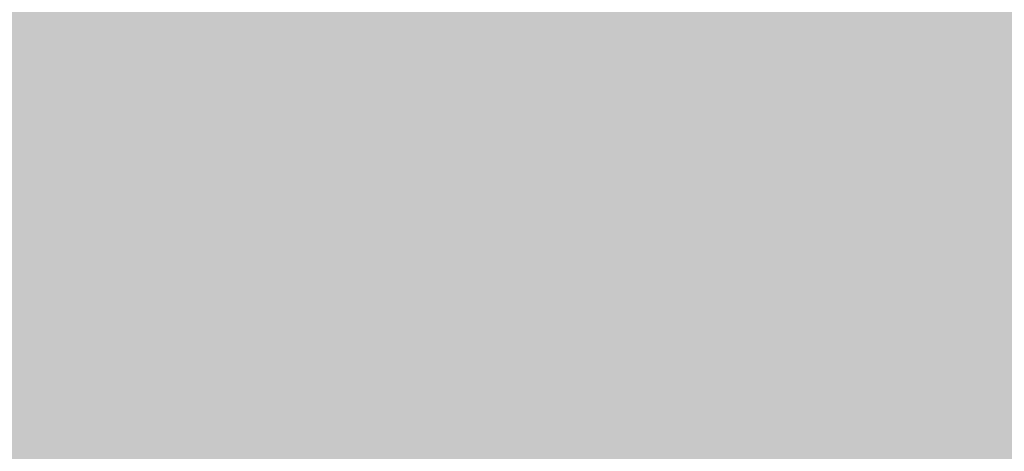
# Model space of a CAD drawing. Units: inches. Extents: x 2083 to 3317, y 1141 to 2115.
# Tile 148 of 256: x 3126.92826 to 3126.94671, y 1263.26594 to 1263.27402. Entities that reach past the tile are written whole.
import ezdxf

# ---------------------------------------------------------------- set-up
doc = ezdxf.new("R2010")
doc.units = ezdxf.units.IN
doc.layers.add('A-ANNO-DIMS', color=2, linetype='Continuous', lineweight=18)
doc.layers.add('A-WALL-PATT', color=251, linetype='Continuous', lineweight=13, true_color=0x636466)
doc.styles.get("Standard").update_dxf_attribs({"font": 'arial.ttf'})
doc.dimstyles.new('ISO-25', dxfattribs={"dimtxt": 12, "dimasz": 12, "dimexe": 1.25, "dimexo": 0.625, "dimtad": 1, "dimlunit": 3, "dimtxsty": 'Standard', "dimcen": 2.5, "dimadec": 0, "dimazin": 0, "dimtfac": 1, "dimtmove": 0, "dimatfit": 3, "dimfxl": 1, "dimarcsym": 0})

# ---------------------------------------------------------------- blocks, each defined once
blk = doc.blocks.new('*D26')
at = {"layer": 'A-ANNO-DIMS', "color": 0, "lineweight": -2, "transparency": 16777216}
for p, q in [((3088.985844, 1274.915092), (3088.985844, 1270.951963)), ((3111.240037, 1274.915092), (3111.240037, 1270.951963)), ((3076.985844, 1272.201963), (2840.262447, 1272.201963)), ((3111.240037, 1272.201963), (3088.985844, 1272.201963)), ((3123.240037, 1272.201963), (3135.240037, 1272.201963))]:
    blk.add_line(p, q, dxfattribs=at)
at = {"layer": 'A-ANNO-DIMS', "color": 0, "transparency": 16777216}
for points in [[(3076.985844, 1274.201963), (3076.985844, 1270.201963), (3088.985844, 1272.201963)], [(3123.240037, 1274.201963), (3123.240037, 1270.201963), (3111.240037, 1272.201963)]]:
    blk.add_solid(points, dxfattribs=at)
at = {"layer": 'Defpoints', "color": 0, "transparency": 16777216}
for p in [(3088.985844, 1275.540092), (3111.240037, 1275.540092), (3088.985844, 1272.201963)]:
    blk.add_point(p, dxfattribs=at)
at = {"layer": 'A-ANNO-DIMS', "color": 0, "transparency": 16777216, "insert": (2952.624146, 1279.031602), "char_height": 12, "attachment_point": 5}
blk.add_mtext('NIGHTSTAND 1\'-10 1/2" TYP.', dxfattribs=at)
blk = doc.blocks.new('*D27')
at = {"layer": 'A-ANNO-DIMS', "color": 0, "lineweight": -2, "transparency": 16777216}
for p, q in [((3114.578165, 1309.794285), (3114.578165, 1321.794285)), ((3111.865037, 1297.794285), (3115.828165, 1297.794285)), ((3114.578165, 1297.794285), (3114.578165, 1275.540092)), ((3111.865037, 1275.540092), (3115.828165, 1275.540092)), ((3114.578165, 1263.540092), (3114.578165, 1140.988591))]:
    blk.add_line(p, q, dxfattribs=at)
at = {"layer": 'A-ANNO-DIMS', "color": 0, "transparency": 16777216}
for points in [[(3112.578165, 1309.794285), (3116.578165, 1309.794285), (3114.578165, 1297.794285)], [(3112.578165, 1263.540092), (3116.578165, 1263.540092), (3114.578165, 1275.540092)]]:
    blk.add_solid(points, dxfattribs=at)
at = {"layer": 'Defpoints', "color": 0, "transparency": 16777216}
for p in [(3111.240037, 1297.794285), (3111.240037, 1275.540092), (3114.578165, 1275.540092)]:
    blk.add_point(p, dxfattribs=at)
at = {"layer": 'A-ANNO-DIMS', "color": 0, "transparency": 16777216, "insert": (3107.748527, 1196.264342), "char_height": 12, "attachment_point": 5, "rotation": 90}
blk.add_mtext('1\'-10 1/2" TYP.', dxfattribs=at)

msp = doc.modelspace()

# ---------------------------------------------------------------- hatches: boundary and pattern name
at = {"layer": 'A-WALL-PATT'}
h = msp.add_hatch(color=256, dxfattribs=at)
h.dxf.hatch_style = 1
h.paths.add_polyline_path([(3126.959783, 2020.76136), (2748.959783, 2020.76136), (2604.959783, 2020.76136), (2226.959783, 2020.76136), (2226.959783, 1702.76136), (2466.959783, 1702.76136), (2466.959783, 1582.76136), (2418.959783, 1582.76136), (2418.959783, 1477.76136), (2226.959783, 1477.76136), (2226.959783, 1263.26136), (2544.959783, 1263.26136), (2544.959783, 1411.76136), (2604.959783, 1411.76136), (2685.959783, 1411.76136), (2685.959783, 1420.76136), (2604.959783, 1420.76136), (2604.959783, 1573.76136), (2604.959783, 1702.76136), (2604.959783, 2011.76136), (2748.959783, 2011.76136), (2748.959783, 1702.76136), (2862.959783, 1702.76136), (2862.959783, 1621.76136), (2871.959783, 1621.76136), (2871.959783, 1702.76136), (2883.959783, 1702.76136), (2883.959783, 1706.939459, -0.026459), (2883.959783, 1711.76136), (2757.959783, 1711.76136), (2757.959783, 1807.76136), (2787.959783, 1807.76136), (2787.959783, 1812.26136), (2757.959783, 1812.26136), (2757.959783, 2011.76136), (2877.959783, 2011.76136), (2877.959783, 1812.26136), (2847.959783, 1812.26136), (2847.959783, 1807.76136), (2889.835742, 1807.76136), (2889.835742, 1812.26136), (2882.459783, 1812.26136), (2882.459783, 2011.76136), (3117.959783, 2011.76136), (3117.959783, 1812.26136), (2937.835742, 1812.26136), (2937.835742, 1807.76136), (2995.709783, 1807.76136), (2995.709783, 1796.117666), (3000.209783, 1796.117666), (3000.209783, 1807.76136), (3117.959783, 1807.76136), (3117.959783, 1711.76136), (3000.209783, 1711.76136), (3000.209783, 1760.117666), (2998.572705, 1760.117666, -0.020711), (2995.709783, 1760.117666), (2995.709783, 1711.76136), (2931.959783, 1711.76136), (2931.959783, 1702.76136), (3126.959783, 1702.76136)])
h.paths.add_polyline_path([(2471.459783, 2011.76136), (2471.459783, 1810.01136), (2462.716936, 1810.01136), (2462.716936, 1805.51136), (2505.959783, 1805.51136), (2505.959783, 1810.01136), (2475.959783, 1810.01136), (2475.959783, 2011.76136), (2595.959783, 2011.76136), (2595.959783, 1810.01136), (2565.959783, 1810.01136), (2565.959783, 1805.51136), (2595.959783, 1805.51136), (2595.959783, 1711.76136), (2235.959783, 1711.76136), (2235.959783, 1805.51136), (2353.709783, 1805.51136), (2353.709783, 1796.054162), (2358.209783, 1796.054162), (2358.209783, 1805.51136), (2414.716936, 1805.51136), (2414.716936, 1810.01136), (2235.959783, 1810.01136), (2235.959783, 2011.76136)], flags=16)
h.paths.add_polyline_path([(2270.204734, 1994.610008), (2270.204734, 1970.610008), (2246.204734, 1970.610008), (2246.204734, 1994.610008)], flags=0)
edge = h.paths.add_edge_path(flags=0)
edge.add_ellipse((2332.027391, 1899.798176), major_axis=(-3.042994, 3.042994), ratio=0.16825245, start_angle=-161.332166, end_angle=-156.307114, ccw=False)
edge.add_ellipse((2333.082037, 1898.74353), major_axis=(-1.054646, 1.054646), ratio=0.4535321, start_angle=-123.371019, end_angle=-94.159107)
edge = h.paths.add_edge_path(flags=0)
edge.add_ellipse((2332.027391, 1968.87629), major_axis=(3.042994, 3.042994), ratio=0.16825245, start_angle=18.667834, end_angle=23.692886)
edge.add_spline(control_points=[(2332.925596, 1970.691105), (2332.226768, 1970.3361), (2330.893709, 1969.658905), (2328.41308, 1970.932138), (2327.203934, 1967.748712), (2324.709596, 1969.955589), (2322.532822, 1967.012354), (2320.012846, 1971.295812), (2317.680308, 1968.157845), (2316.040526, 1967.102047), (2315.426904, 1966.809602)], knot_values=[0, 0, 0, 0, 2.267059, 4.324559, 6.685584, 8.878641, 11.121502, 14.300359, 17.755284, 19.732645, 19.732645, 19.732645, 19.732645], degree=3, periodic=0)
edge.add_ellipse((2332.027391, 1968.87629), major_axis=(3.042994, 3.042994), ratio=0.16825245, start_angle=18.667834, end_angle=23.692886, ccw=False)
edge.add_ellipse((2333.082037, 1969.930936), major_axis=(1.054646, 1.054646), ratio=0.4535321, start_angle=56.628981, end_angle=85.840893, ccw=False)
edge = h.paths.add_edge_path(flags=0)
edge.add_spline(control_points=[(2296.428287, 1967.987908), (2293.627804, 1965.336314), (2287.703624, 1959.727094), (2299.74386, 1949.995699), (2294.532591, 1935.668528), (2290.573228, 1920.603512), (2293.394124, 1909.973691), (2296.185407, 1904.966543)], knot_values=[0.099185, 0.099185, 0.099185, 0.099185, 0.345301, 0.619822, 0.982653, 1.386093, 1.810555, 1.810555, 1.810555, 1.810555], degree=3, periodic=0)
edge.add_spline(control_points=[(2296.185407, 1904.966543), (2297.383582, 1902.6193), (2298.000969, 1901.949312), (2298.55297, 1901.468155)], knot_values=[0.006246, 0.006246, 0.006246, 0.006246, 0.055476, 0.055476, 0.055476, 0.055476], degree=3, periodic=0)
edge.add_spline(control_points=[(2298.55297, 1901.468155), (2297.258612, 1900.923224), (2295.225294, 1900.232126), (2293.060229, 1900.614205), (2292.101423, 1900.788415), (2292.089578, 1900.790568)], knot_values=[0.312835, 0.312835, 0.312835, 0.312835, 0.40178, 0.474987, 0.475903, 0.475903, 0.475903, 0.475903], degree=3, periodic=0)
edge.add_arc((2292.793646, 1904.664109), 3.937008, 215.420897, 259.698179, ccw=False)
edge.add_spline(control_points=[(2289.585314, 1902.382304), (2289.476652, 1902.535087), (2289.36848, 1902.688035), (2289.260865, 1902.84117)], knot_values=[0.102872, 0.102872, 0.102872, 0.102872, 0.116896, 0.116896, 0.116896, 0.116896], degree=3, periodic=0)
edge.add_spline(control_points=[(2289.260865, 1902.84117), (2288.686604, 1902.550192), (2287.640048, 1902.019902), (2285.881337, 1901.873954), (2283.852972, 1901.504352), (2281.719987, 1899.710538), (2278.466991, 1899.492942), (2276.157136, 1901.883202), (2272.258953, 1899.804071), (2267.777605, 1901.843183), (2262.243882, 1900.184033), (2257.414927, 1901.782061), (2254.318374, 1900.72612), (2253.178285, 1900.337343)], knot_values=[0, 0, 0, 0, 1.907977, 3.477176, 5.261074, 7.972851, 11.680248, 13.717921, 16.939592, 22.789562, 27.502503, 33.595215, 37.145618, 37.145618, 37.145618, 37.145618], degree=3, periodic=0)
edge.add_line((2253.178285, 1900.337343), (2250.24424, 1902.84117))
edge.add_line((2250.24424, 1902.84117), (2250.24424, 1965.833296))
edge.add_line((2250.24424, 1965.833296), (2253.178285, 1968.337123))
edge.add_spline(control_points=[(2253.178285, 1968.337123), (2254.318374, 1967.948346), (2257.414927, 1966.892405), (2262.243882, 1968.490433), (2267.777605, 1966.831283), (2271.52673, 1968.537217), (2273.875914, 1967.828289), (2274.206701, 1967.727642)], knot_values=[0, 0, 0, 0, 0.09018, 0.244935, 0.364644, 0.513233, 0.537855, 0.537855, 0.537855, 0.537855], degree=3, periodic=0)
edge.add_arc((2274.352887, 1963.793349), 3.937008, 72.051134, 92.127949, ccw=False)
edge.add_arc((2281.296933, 1985.230003), 18.596298, 252.0511336, 288.5657217)
edge.add_arc((2292.316717, 1956.02888), 12.646081, 71.0267879, 113.7782184, ccw=False)
edge = h.paths.add_edge_path(flags=0)
edge.add_spline(control_points=[(2274.899415, 1951.856195), (2275.066156, 1951.616592), (2275.232687, 1951.376588), (2275.397987, 1951.135855)], knot_values=[1.409916, 1.409916, 1.409916, 1.409916, 1.43159, 1.43159, 1.43159, 1.43159], degree=3, periodic=0)
edge.add_spline(control_points=[(2275.397987, 1951.135855), (2275.792106, 1950.561885), (2276.179231, 1949.983774), (2276.545546, 1949.397103)], knot_values=[1.358238, 1.358238, 1.358238, 1.358238, 1.409916, 1.409916, 1.409916, 1.409916], degree=3, periodic=0)
edge.add_line((2276.545546, 1949.397103), (2277.437289, 1947.862185))
edge.add_spline(control_points=[(2277.437289, 1947.862185), (2276.303834, 1945.673115), (2274.639698, 1942.426882), (2274.631615, 1938.0939), (2272.799124, 1930.85155), (2274.356426, 1943.897046), (2275.947681, 1947.923356), (2276.545546, 1949.397103)], knot_values=[0.005632, 0.005632, 0.005632, 0.005632, 0.186014, 0.266002, 0.357087, 0.59639, 0.739732, 0.739732, 0.739732, 0.739732], degree=3, periodic=0)
edge.add_spline(control_points=[(2276.545546, 1949.397103), (2276.179231, 1949.983774), (2275.792106, 1950.561885), (2275.397987, 1951.135855)], knot_values=[1.358238, 1.358238, 1.358238, 1.358238, 1.409916, 1.409916, 1.409916, 1.409916], degree=3, periodic=0)
edge.add_spline(control_points=[(2275.397987, 1951.135855), (2274.9425, 1950.080452), (2274.20776, 1948.025272), (2273.934602, 1944.851477), (2272.468534, 1937.627489), (2273.466216, 1945.696466), (2274.700615, 1951.059472), (2274.899415, 1951.856195)], knot_values=[0.104364, 0.104364, 0.104364, 0.104364, 0.189636, 0.269624, 0.36071, 0.600013, 0.644622, 0.644622, 0.644622, 0.644622], degree=3, periodic=0)
h.paths.add_polyline_path([(2269.167514, 1963.127573, -0.357527), (2268.170633, 1960.97637, -0.092561), (2268.170633, 1939.436325, -0.357527), (2269.167514, 1937.285122, -0.357527), (2267.01631, 1938.282002, -0.164785), (2254.685581, 1938.282002, -0.357527), (2252.534378, 1937.285122, -0.357527), (2253.531259, 1939.436325, -0.092561), (2253.531259, 1960.97637, -0.357527), (2252.534378, 1963.127573, -0.357527), (2254.685581, 1962.130692, -0.164785), (2267.01631, 1962.130692, -0.357527)], flags=0)
h.paths.add_polyline_path([(2248.874068, 1967.8018), (2248.874068, 1957.02771), (2249.457783, 1957.02771), (2249.457783, 1911.646756), (2248.874068, 1911.646756), (2248.874068, 1900.872666), (2246.511863, 1900.872666, 0.197327), (2244.149658, 1902.456873), (2244.149658, 1966.217592, 0.197327), (2246.511863, 1967.8018)], flags=0)
h.paths.add_polyline_path([(2269.167514, 1931.389344, -0.357527), (2268.170633, 1929.238141, -0.092561), (2268.170633, 1907.698096, -0.357527), (2269.167514, 1905.546893, -0.357527), (2267.01631, 1906.543774, -0.164785), (2254.685581, 1906.543774, -0.357527), (2252.534378, 1905.546893, -0.357527), (2253.531259, 1907.698096, -0.092561), (2253.531259, 1929.238141, -0.357527), (2252.534378, 1931.389344, -0.357527), (2254.685581, 1930.392463, -0.164785), (2267.01631, 1930.392463, -0.357527)], flags=0)
edge = h.paths.add_edge_path(flags=0)
edge.add_spline(control_points=[(2276.196858, 1906.723702), (2276.168144, 1909.028928), (2276.114049, 1913.371852), (2270.598417, 1924.924978), (2273.905175, 1919.012779), (2275.921711, 1916.262063), (2275.47457, 1912.402149), (2277.257874, 1910.380621), (2276.696044, 1908.225036), (2276.646218, 1906.813023), (2276.617825, 1906.008407)], knot_values=[0, 0, 0, 0, 8.61026, 16.221274, 18.843057, 23.804898, 27.440828, 29.356102, 31.203478, 33.650687, 33.650687, 33.650687, 33.650687], degree=3, periodic=0)
edge.add_spline(control_points=[(2276.617825, 1906.008407), (2276.623313, 1905.624144), (2276.497738, 1904.628661), (2275.441779, 1903.854725), (2274.937314, 1903.08045), (2274.85908, 1902.84117)], knot_values=[0.156488, 0.156488, 0.156488, 0.156488, 0.184398, 0.231376, 0.250598, 0.250598, 0.250598, 0.250598], degree=3, periodic=0)
edge.add_line((2274.85908, 1902.84117), (2276.50598, 1902.84117))
edge.add_spline(control_points=[(2276.50598, 1902.84117), (2276.788308, 1903.08494), (2277.665071, 1904.125196), (2278.249538, 1904.340738), (2277.653872, 1908.527387), (2278.15567, 1906.227808), (2278.100464, 1905.285948), (2278.846675, 1904.069005), (2277.856785, 1903.414948), (2277.874191, 1902.99105), (2277.903562, 1902.84117)], knot_values=[0.059574, 0.059574, 0.059574, 0.059574, 0.080753, 0.103741, 0.16972, 0.176036, 0.207137, 0.240474, 0.262341, 0.27366, 0.27366, 0.27366, 0.27366], degree=3, periodic=0)
edge.add_line((2277.903562, 1902.84117), (2280.029825, 1902.84117))
edge.add_spline(control_points=[(2280.029825, 1902.84117), (2279.888221, 1903.088398), (2279.499257, 1903.981551), (2280.152284, 1905.939349), (2278.103615, 1909.657757), (2279.762395, 1907.185285), (2280.3279, 1904.874861), (2280.485109, 1903.48959), (2281.463269, 1903.249432), (2281.758343, 1902.936497), (2281.834036, 1902.84117)], knot_values=[0.013856, 0.013856, 0.013856, 0.013856, 0.034874, 0.088867, 0.107879, 0.126738, 0.158714, 0.193757, 0.217487, 0.226722, 0.226722, 0.226722, 0.226722], degree=3, periodic=0)
edge.add_spline(control_points=[(2281.834036, 1902.84117), (2281.787535, 1902.826703), (2281.647022, 1902.782988), (2281.395527, 1902.85949), (2281.088077, 1902.985242), (2280.720683, 1903.060902), (2280.333451, 1903.025726), (2280.124767, 1902.898879), (2280.029825, 1902.84117)], knot_values=[0, 0, 0, 0, 0.14413, 0.435517, 0.749276, 1.153046, 1.548371, 1.878348, 1.878348, 1.878348, 1.878348], degree=3, periodic=0)
edge.add_line((2280.029825, 1902.84117), (2277.903562, 1902.84117))
edge.add_spline(control_points=[(2277.903562, 1902.84117), (2277.892855, 1902.795855), (2277.865396, 1902.679637), (2277.607479, 1902.687483), (2277.27405, 1902.8007), (2276.837921, 1902.619775), (2276.583807, 1902.789261), (2276.50598, 1902.84117)], knot_values=[0, 0, 0, 0, 0.127189, 0.326199, 0.628009, 1.24357, 1.515331, 1.515331, 1.515331, 1.515331], degree=3, periodic=0)
edge.add_line((2276.50598, 1902.84117), (2274.85908, 1902.84117))
edge.add_spline(control_points=[(2274.85908, 1902.84117), (2274.814437, 1902.898587), (2274.72513, 1903.013446), (2274.493477, 1903.118968), (2274.244285, 1902.960539), (2273.937121, 1903.184942), (2273.614039, 1902.983143), (2273.408316, 1902.883045), (2273.322254, 1902.84117)], knot_values=[0, 0, 0, 0, 0.21843, 0.436957, 0.687977, 0.990379, 1.398396, 1.69185, 1.69185, 1.69185, 1.69185], degree=3, periodic=0)
edge.add_spline(control_points=[(2273.322254, 1902.84117), (2273.61674, 1903.445692), (2274.273998, 1904.538253), (2276.027239, 1904.573702), (2276.206963, 1906.583637), (2276.196858, 1906.723702)], knot_values=[0.012227, 0.012227, 0.012227, 0.012227, 0.059472, 0.106218, 0.134458, 0.134458, 0.134458, 0.134458], degree=3, periodic=0)
h.paths.add_polyline_path([(2270.776054, 1897.789828), (2270.776054, 1873.789828), (2246.776054, 1873.789828), (2246.776054, 1897.789828)], flags=0)
h.paths.add_polyline_path([(2353.709783, 1760.005059), (2353.709783, 1760.054162), (2358.209783, 1760.054162, -0.033729)], flags=0)
h.paths.add_polyline_path([(2321.819119, 1737.529186), (2341.995327, 1737.529186, -0.414214), (2343.203273, 1736.321241), (2343.203273, 1721.020596, -0.414214), (2341.995327, 1719.812651), (2321.819119, 1719.812651, -0.414214), (2320.611173, 1721.020596), (2320.611173, 1736.321241, -0.414214)], flags=0)
h.paths.add_polyline_path([(2324.23501, 1736.321241), (2339.579436, 1736.321241, -0.414214), (2341.995327, 1733.905349), (2341.995327, 1725.44973, -0.414214), (2339.579436, 1723.033839), (2333.680588, 1723.033839), (2333.845317, 1722.045467, -0.870646), (2335.425399, 1721.825893, -0.767327), (2333.922694, 1721.423245), (2331.291024, 1721.423245, -0.767327), (2329.788319, 1721.825893, -0.870646), (2331.368401, 1722.045467), (2331.53313, 1723.033839), (2324.23501, 1723.033839, -0.414214), (2321.819119, 1725.44973), (2321.819119, 1733.905349, -0.414214)], flags=0)
h.paths.add_polyline_path([(2570.483789, 1928.615444), (2589.683789, 1928.615444), (2590.168829, 1928.615444), (2590.168829, 1904.993397), (2570.483789, 1904.993397)], flags=0)
h.paths.add_polyline_path([(2574.447324, 1927.263822, -1), (2572.828836, 1927.263822, -1)], flags=0)
h.paths.add_polyline_path([(2573.089867, 1926.940877), (2573.925032, 1927.776042), (2574.147743, 1927.553332), (2573.312577, 1926.718166)], flags=0)
h.paths.add_polyline_path([(2578.779065, 1919.729618, -1), (2571.591663, 1919.729618, -1)], flags=0)
h.paths.add_polyline_path([(2578.385364, 1919.729618, -1), (2571.985364, 1919.729618, -1)], flags=0)
h.paths.add_polyline_path([(2331.595764, 1729.476216, -1), (2333.617954, 1729.476216, -1)], flags=0)
h.paths.add_polyline_path([(2578.034228, 1927.263822, -1), (2576.41574, 1927.263822, -1)], flags=0)
h.paths.add_polyline_path([(2576.688851, 1927.531089), (2576.911562, 1927.753799), (2577.746728, 1926.918634), (2577.524017, 1926.695923)], flags=0)
h.paths.add_polyline_path([(2578.139065, 1909.859539, -1), (2572.231663, 1909.859539, -1)], flags=0)
h.paths.add_polyline_path([(2577.745364, 1909.859539, -1), (2572.625364, 1909.859539, -1)], flags=0)
h.paths.add_polyline_path([(2583.797718, 1927.263822, -1), (2582.179229, 1927.263822, -1)], flags=0)
h.paths.add_polyline_path([(2582.718649, 1927.753799), (2583.553814, 1926.918634), (2583.331103, 1926.695923), (2582.495938, 1927.531089)], flags=0)
h.paths.add_polyline_path([(2582.495938, 1927.531089), (2582.718649, 1927.753799), (2583.553814, 1926.918634), (2583.331103, 1926.695923)], flags=0)
h.paths.add_polyline_path([(2587.739065, 1920.529618, -1), (2581.831663, 1920.529618, -1)], flags=0)
h.paths.add_polyline_path([(2587.345364, 1920.529618, -1), (2582.225364, 1920.529618, -1)], flags=0)
h.paths.add_polyline_path([(2587.384622, 1927.263822, -1), (2585.766133, 1927.263822, -1)], flags=0)
h.paths.add_polyline_path([(2586.081993, 1926.980247), (2586.917158, 1927.815412), (2587.139869, 1927.592702), (2586.304703, 1926.757536)], flags=0)
h.paths.add_polyline_path([(2588.379065, 1910.659539, -1), (2581.191663, 1910.659539, -1)], flags=0)
h.paths.add_polyline_path([(2587.985364, 1910.659539, -1), (2581.585364, 1910.659539, -1)], flags=0)
h.paths.add_polyline_path([(2417.167729, 1729.477895), (2437.343937, 1729.477895, -0.414214), (2438.551883, 1728.26995), (2438.551883, 1712.969306, -0.414214), (2437.343937, 1711.76136), (2417.167729, 1711.76136, -0.414214), (2415.959783, 1712.969306), (2415.959783, 1728.26995, -0.414214)], flags=0)
h.paths.add_polyline_path([(2419.58362, 1728.26995), (2434.928046, 1728.26995, -0.414214), (2437.343937, 1725.854059), (2437.343937, 1717.39844, -0.414214), (2434.928046, 1714.982548), (2429.029199, 1714.982548), (2429.193927, 1713.994176, -0.870646), (2430.774009, 1713.774603, -0.767327), (2429.271304, 1713.371954), (2426.639634, 1713.371954, -0.767327), (2425.136929, 1713.774603, -0.870646), (2426.717011, 1713.994176), (2426.88174, 1714.982548), (2419.58362, 1714.982548, -0.414214), (2417.167729, 1717.39844), (2417.167729, 1725.854059, -0.414214)], flags=0)
h.paths.add_polyline_path([(2419.58362, 1728.26995), (2434.928046, 1728.26995, -0.414214), (2437.343937, 1725.854059), (2437.343937, 1717.39844, -0.414214), (2434.928046, 1714.982548), (2429.029199, 1714.982548), (2428.358118, 1719.009034), (2427.552821, 1719.009034), (2426.88174, 1714.982548), (2419.58362, 1714.982548, -0.414214), (2417.167729, 1717.39844), (2417.167729, 1725.854059, -0.414214)], flags=0)
h.paths.add_polyline_path([(2426.944374, 1721.424925, -1), (2428.966564, 1721.424925, -1)], flags=0)
h.paths.add_polyline_path([(2475.959783, 1702.76136), (2595.959783, 1702.76136), (2595.959783, 1582.76136), (2475.959783, 1582.76136)], flags=16)
h.paths.add_polyline_path([(2427.959783, 1573.76136), (2595.959783, 1573.76136), (2595.959783, 1468.76136), (2595.959783, 1420.76136), (2384.459783, 1420.76136), (2384.459783, 1468.76136), (2427.959783, 1468.76136)], flags=16)
h.paths.add_polyline_path([(2379.959783, 1468.76136), (2379.959783, 1420.76136), (2235.959783, 1420.76136), (2235.959783, 1468.76136)], flags=16)
h.paths.add_polyline_path([(2317.815996, 1466.695767), (2337.992205, 1466.695767, -0.414214), (2339.20015, 1465.487821), (2339.20015, 1450.187177, -0.414214), (2337.992205, 1448.979232), (2317.815996, 1448.979232, -0.414214), (2316.608051, 1450.187177), (2316.608051, 1465.487821, -0.414214)], flags=0)
h.paths.add_polyline_path([(2320.231887, 1465.487821), (2335.576313, 1465.487821, -0.414214), (2337.992205, 1463.07193), (2337.992205, 1454.616311, -0.414214), (2335.576313, 1452.20042), (2329.677466, 1452.20042), (2329.842195, 1451.212047, -0.870646), (2331.422276, 1450.992474, -0.767327), (2329.919571, 1450.589826), (2327.287902, 1450.589826, -0.767327), (2325.785197, 1450.992474, -0.870646), (2327.365278, 1451.212047), (2327.530007, 1452.20042), (2320.231887, 1452.20042, -0.414214), (2317.815996, 1454.616311), (2317.815996, 1463.07193, -0.414214)], flags=0)
h.paths.add_polyline_path([(2320.231887, 1465.487821), (2335.576313, 1465.487821, -0.414214), (2337.992205, 1463.07193), (2337.992205, 1454.616311, -0.414214), (2335.576313, 1452.20042), (2329.677466, 1452.20042), (2329.006385, 1456.226905), (2328.201088, 1456.226905), (2327.530007, 1452.20042), (2320.231887, 1452.20042, -0.414214), (2317.815996, 1454.616311), (2317.815996, 1463.07193, -0.414214)], flags=0)
h.paths.add_polyline_path([(2327.592641, 1458.642796, -1), (2329.614832, 1458.642796, -1)], flags=0)
h.paths.add_polyline_path([(2244.411744, 1433.340453), (2241.920945, 1433.340453, -0.414214), (2240.017856, 1435.243542), (2240.017856, 1440.952808, -0.414211), (2241.920925, 1442.855897), (2244.411744, 1442.855897, -1.976472)], flags=0)
h.paths.add_polyline_path([(2245.356888, 1434.397536, -0.414214), (2245.356888, 1441.798814, -2.144098)], flags=0)
h.paths.add_polyline_path([(2535.959783, 1416.26136), (2535.959783, 1272.26136), (2235.959783, 1272.26136), (2235.959783, 1416.26136)], flags=16)
h.paths.add_polyline_path([(2260.119561, 1384.292841), (2260.119561, 1362.038649), (2237.865369, 1362.038649), (2237.865369, 1384.292841)], flags=0)
edge = h.paths.add_edge_path(flags=0)
edge.add_line((2318.251847, 1362.093298), (2318.145797, 1362.000973))
edge.add_ellipse((2317.445116, 1360.431044), major_axis=(2.82164, 2.82164), ratio=0.16825245, start_angle=18.667834, end_angle=20.948127, ccw=False)
edge.add_ellipse((2318.423045, 1361.408974), major_axis=(0.977929, 0.977929), ratio=0.4535321, start_angle=56.628981, end_angle=70.226201, ccw=False)
edge = h.paths.add_edge_path(flags=0)
edge.add_line((2319.10737, 1295.571078), (2319.015044, 1295.677128))
edge.add_ellipse((2317.445116, 1296.377809), major_axis=(-2.82164, 2.82164), ratio=0.16825245, start_angle=-161.332166, end_angle=-159.051873, ccw=False)
edge.add_ellipse((2318.423045, 1295.39988), major_axis=(-0.977929, 0.977929), ratio=0.4535321, start_angle=-123.371019, end_angle=-109.773799)
edge = h.paths.add_edge_path(flags=0)
edge.add_spline(control_points=[(2284.210349, 1301.170219), (2284.580688, 1300.444719), (2284.891189, 1299.892024), (2285.159553, 1299.461018)], knot_values=[0.039066, 0.039066, 0.039066, 0.039066, 0.055476, 0.055476, 0.055476, 0.055476], degree=3, periodic=0)
edge.add_line((2285.159553, 1299.461018), (2284.210349, 1301.170219))
edge = h.paths.add_edge_path(flags=0)
edge.add_line((2280.412458, 1297.298013), (2283.369991, 1297.036122))
edge.add_line((2283.369991, 1297.036122), (2286.40569, 1297.92631))
edge.add_spline(control_points=[(2286.40569, 1297.92631), (2285.305487, 1297.463119), (2284.344777, 1297.129151), (2283.369991, 1297.036122)], knot_values=[0.394369, 0.394369, 0.394369, 0.394369, 0.475903, 0.475903, 0.475903, 0.475903], degree=3, periodic=0)
edge.add_spline(control_points=[(2283.369991, 1297.036122), (2283.28139, 1297.027666), (2282.316289, 1296.957336), (2281.312502, 1297.134479), (2280.423441, 1297.296016), (2280.412458, 1297.298013)], knot_values=[0.312835, 0.312835, 0.312835, 0.312835, 0.320246, 0.393453, 0.394369, 0.394369, 0.394369, 0.394369], degree=3, periodic=0)
edge = h.paths.add_edge_path(flags=0)
edge.add_line((2284.435561, 1359.607285), (2280.446291, 1355.328047))
edge.add_line((2280.446291, 1355.328047), (2279.579987, 1351.017754))
edge.add_line((2279.579987, 1351.017754), (2282.412974, 1346.580433))
edge.add_spline(control_points=[(2282.412974, 1346.580433), (2283.153331, 1345.589236), (2284.252896, 1344.028897), (2284.801037, 1342.387167), (2284.935162, 1341.805544)], knot_values=[1.240098, 1.240098, 1.240098, 1.240098, 1.332892, 1.382712, 1.382712, 1.382712, 1.382712], degree=3, periodic=0)
edge.add_spline(control_points=[(2284.935162, 1341.805544), (2285.319108, 1340.1406), (2285.233029, 1338.409204), (2284.909938, 1336.654122)], knot_values=[1.097484, 1.097484, 1.097484, 1.097484, 1.240098, 1.240098, 1.240098, 1.240098], degree=3, periodic=0)
edge.add_spline(control_points=[(2284.909938, 1336.654122), (2284.586848, 1334.89904), (2284.026745, 1333.120272), (2283.462644, 1331.360585)], knot_values=[0.95487, 0.95487, 0.95487, 0.95487, 1.097484, 1.097484, 1.097484, 1.097484], degree=3, periodic=0)
edge.add_line((2283.462644, 1331.360585), (2281.890376, 1326.153357))
edge.add_line((2281.890376, 1326.153357), (2280.756259, 1321.056089))
edge.add_line((2280.756259, 1321.056089), (2280.299205, 1316.001977))
edge.add_line((2280.299205, 1316.001977), (2280.715933, 1310.950068))
edge.add_line((2280.715933, 1310.950068), (2282.028094, 1305.972137))
edge.add_line((2282.028094, 1305.972137), (2284.210349, 1301.170219))
edge.add_spline(control_points=[(2284.210349, 1301.170219), (2283.340731, 1302.730185), (2282.611904, 1304.336493), (2282.028094, 1305.972137)], knot_values=[0.099185, 0.099185, 0.099185, 0.099185, 0.241799, 0.241799, 0.241799, 0.241799], degree=3, periodic=0)
edge.add_spline(control_points=[(2282.028094, 1305.972137), (2281.444283, 1307.60778), (2281.005489, 1309.272759), (2280.715933, 1310.950068)], knot_values=[0.241799, 0.241799, 0.241799, 0.241799, 0.384413, 0.384413, 0.384413, 0.384413], degree=3, periodic=0)
edge.add_spline(control_points=[(2280.715933, 1310.950068), (2280.433241, 1312.587613), (2280.289386, 1314.276959), (2280.298894, 1315.962032), (2280.299205, 1316.001977)], knot_values=[0.384413, 0.384413, 0.384413, 0.384413, 0.523647, 0.527028, 0.527028, 0.527028, 0.527028], degree=3, periodic=0)
edge.add_spline(control_points=[(2280.299205, 1316.001977), (2280.312326, 1317.686955), (2280.477871, 1319.367926), (2280.756259, 1321.056089)], knot_values=[0.527028, 0.527028, 0.527028, 0.527028, 0.669642, 0.669642, 0.669642, 0.669642], degree=3, periodic=0)
edge.add_spline(control_points=[(2280.756259, 1321.056089), (2281.034648, 1322.744252), (2281.42588, 1324.439608), (2281.890376, 1326.153357)], knot_values=[0.669642, 0.669642, 0.669642, 0.669642, 0.812256, 0.812256, 0.812256, 0.812256], degree=3, periodic=0)
edge.add_spline(control_points=[(2281.890376, 1326.153357), (2282.264383, 1327.533251), (2282.78787, 1329.26181), (2283.352751, 1331.01778), (2283.462644, 1331.360585)], knot_values=[0.812256, 0.812256, 0.812256, 0.812256, 0.927087, 0.95487, 0.95487, 0.95487, 0.95487], degree=3, periodic=0)
edge.add_line((2283.462644, 1331.360585), (2284.909938, 1336.654122))
edge.add_line((2284.909938, 1336.654122), (2284.935162, 1341.805544))
edge.add_line((2284.935162, 1341.805544), (2282.412974, 1346.580433))
edge.add_spline(control_points=[(2282.412974, 1346.580433), (2281.275127, 1348.103792), (2280.078447, 1349.570318), (2279.579987, 1351.017754)], knot_values=[1.382712, 1.382712, 1.382712, 1.382712, 1.525326, 1.525326, 1.525326, 1.525326], degree=3, periodic=0)
edge.add_spline(control_points=[(2279.579987, 1351.017754), (2279.443282, 1351.414721), (2279.136312, 1352.856922), (2279.73519, 1354.290385), (2280.446291, 1355.328047)], knot_values=[1.525326, 1.525326, 1.525326, 1.525326, 1.564439, 1.667941, 1.667941, 1.667941, 1.667941], degree=3, periodic=0)
edge.add_spline(control_points=[(2280.446291, 1355.328047), (2281.426113, 1356.757835), (2282.930837, 1358.18256), (2284.435561, 1359.607285)], knot_values=[1.667941, 1.667941, 1.667941, 1.667941, 1.810555, 1.810555, 1.810555, 1.810555], degree=3, periodic=0)
edge.add_arc((2280.623075, 1348.518181), 11.72618, 71.0267879, 113.7782184)
edge.add_arc((2270.404892, 1375.595156), 17.243567, 252.0511336, 288.5657217, ccw=False)
edge.add_arc((2263.965969, 1355.717847), 3.650622, 72.051134, 92.127949)
edge.add_arc((2263.965969, 1355.717847), 3.650622, 92.127949, 177.98513)
edge.add_spline(control_points=[(2260.317604, 1355.846199), (2260.260417, 1354.220668), (2260.551278, 1350.186547), (2262.999344, 1346.766251), (2264.472741, 1344.649024)], knot_values=[1.43159, 1.43159, 1.43159, 1.43159, 1.564144, 1.770695, 1.770695, 1.770695, 1.770695], degree=3, periodic=0)
edge.add_line((2264.472741, 1344.649024), (2264.93559, 1343.98253))
edge.add_spline(control_points=[(2263.801044, 1340.248105), (2263.843238, 1340.514088), (2264.067244, 1341.756465), (2264.512693, 1343.002453), (2264.935047, 1343.981083)], knot_values=[0.53657, 0.53657, 0.53657, 0.53657, 0.559349, 0.644622, 0.644622, 0.644622, 0.644622], degree=3, periodic=0)
edge.add_spline(control_points=[(2264.935047, 1343.981083), (2265.117771, 1343.714975), (2265.298875, 1343.447906), (2265.476756, 1343.179365)], knot_values=[1.384077, 1.384077, 1.384077, 1.384077, 1.409916, 1.409916, 1.409916, 1.409916], degree=3, periodic=0)
edge.add_spline(control_points=[(2265.476756, 1343.179365), (2265.654637, 1342.910823), (2265.829296, 1342.64081), (2265.99913, 1342.368812)], knot_values=[1.358238, 1.358238, 1.358238, 1.358238, 1.384077, 1.384077, 1.384077, 1.384077], degree=3, periodic=0)
edge.add_line((2265.99913, 1342.368812), (2266.826006, 1340.945547))
edge.add_spline(control_points=[(2266.826006, 1340.945547), (2268.894401, 1337.089691), (2271.398173, 1325.843001), (2270.516164, 1310.568557), (2275.919376, 1301.860609), (2277.789511, 1299.19945)], knot_values=[0.116896, 0.116896, 0.116896, 0.116896, 0.472987, 1.050969, 1.313793, 1.313793, 1.313793, 1.313793], degree=3, periodic=0)
edge.add_spline(control_points=[(2277.789511, 1299.19945), (2277.839405, 1299.128452), (2277.889428, 1299.057498), (2277.939572, 1298.986584)], knot_values=[0.109884, 0.109884, 0.109884, 0.109884, 0.116896, 0.116896, 0.116896, 0.116896], degree=3, periodic=0)
edge.add_line((2277.939572, 1298.986584), (2277.788849, 1299.199114))
edge.add_spline(control_points=[(2277.788849, 1299.199114), (2277.256582, 1298.929414), (2276.28635, 1298.437902), (2275.039352, 1298.334419), (2274.38333, 1298.238895), (2274.215254, 1298.209338)], knot_values=[33.12187, 33.12187, 33.12187, 33.12187, 35.029056, 36.598255, 37.144827, 37.144827, 37.144827, 37.144827], degree=3, periodic=0)
edge.add_line((2274.215254, 1298.209338), (2273.073147, 1297.892961))
edge.add_spline(control_points=[(2273.073147, 1297.892961), (2272.322936, 1297.579784), (2271.039151, 1296.510508), (2269.248395, 1296.226062), (2268.4231, 1296.374654)], knot_values=[26.532584, 26.532584, 26.532584, 26.532584, 29.198919, 31.839101, 31.839101, 31.839101, 31.839101], degree=3, periodic=0)
edge.add_line((2268.4231, 1296.374654), (2263.878501, 1297.457534))
edge.add_spline(control_points=[(2263.878501, 1297.457534), (2263.556077, 1297.359435), (2261.860306, 1296.838694), (2260.23878, 1297.282407), (2258.933454, 1297.516461)], knot_values=[15.919551, 15.919551, 15.919551, 15.919551, 16.939592, 21.226067, 21.226067, 21.226067, 21.226067], degree=3, periodic=0)
edge.add_line((2258.933454, 1297.516461), (2254.055233, 1297.32901))
edge.add_spline(control_points=[(2254.055233, 1297.32901), (2253.755525, 1297.295815), (2252.113683, 1297.165174), (2250.461869, 1297.544221), (2249.129686, 1297.667882)], knot_values=[5.306517, 5.306517, 5.306517, 5.306517, 6.276435, 10.613034, 10.613034, 10.613034, 10.613034], degree=3, periodic=0)
edge.add_line((2249.129686, 1297.667882), (2244.33165, 1296.877756))
edge.add_line((2244.33165, 1296.877756), (2241.611033, 1299.19945))
edge.add_line((2241.611033, 1299.19945), (2241.611033, 1357.609404))
edge.add_line((2241.611033, 1357.609404), (2244.33165, 1359.931097))
edge.add_line((2244.33165, 1359.931097), (2252.728823, 1359.542692))
edge.add_spline(control_points=[(2252.728823, 1359.542692), (2252.870939, 1359.54644), (2253.30574, 1359.548172), (2253.739845, 1359.514274), (2254.031742, 1359.482426)], knot_values=[0.233291, 0.233291, 0.233291, 0.233291, 0.244935, 0.268927, 0.268927, 0.268927, 0.268927], degree=3, periodic=0)
edge.add_line((2254.031742, 1359.482426), (2259.58719, 1359.41639))
edge.add_spline(control_points=[(2259.58719, 1359.41639), (2260.677068, 1359.628503), (2262.073197, 1359.897003), (2263.523692, 1359.459278), (2263.830417, 1359.365952)], knot_values=[0.422516, 0.422516, 0.422516, 0.422516, 0.513233, 0.537855, 0.537855, 0.537855, 0.537855], degree=3, periodic=0)
edge.add_arc((2263.965969, 1355.717847), 3.650622, 72.051134, 92.127949, ccw=False)
edge.add_arc((2270.404892, 1375.595156), 17.243567, 252.0511336, 288.5657217)
edge.add_arc((2280.623075, 1348.518181), 11.72618, 71.0267879, 113.7782184, ccw=False)
h.paths.add_polyline_path([(2240.34053, 1359.434715), (2240.34053, 1349.444353), (2240.881785, 1349.444353), (2240.881785, 1307.3645), (2240.34053, 1307.3645), (2240.34053, 1297.374138), (2238.150157, 1297.374138, 0.197327), (2235.959783, 1298.843108), (2235.959783, 1357.965746, 0.197327), (2238.150157, 1359.434715)], flags=0)
h.paths.add_polyline_path([(2259.15779, 1355.1005, -0.357527), (2258.233425, 1353.10578, -0.092561), (2258.233425, 1333.132601, -0.357527), (2259.15779, 1331.13788, -0.357527), (2257.16307, 1332.062246, -0.164785), (2245.729302, 1332.062246, -0.357527), (2243.734582, 1331.13788, -0.357527), (2244.658947, 1333.132601, -0.092561), (2244.658947, 1353.10578, -0.357527), (2243.734582, 1355.1005, -0.357527), (2245.729302, 1354.176135, -0.164785), (2257.16307, 1354.176135, -0.357527)], flags=0)
edge = h.paths.add_edge_path(flags=0)
edge.add_line((2265.99913, 1342.368812), (2266.826006, 1340.945547))
edge.add_line((2266.826006, 1340.945547), (2265.307557, 1337.814066))
edge.add_line((2265.307557, 1337.814066), (2264.358232, 1334.652939))
edge.add_line((2264.358232, 1334.652939), (2264.262012, 1333.799705))
edge.add_spline(control_points=[(2264.262012, 1333.799705), (2264.208357, 1333.187055), (2264.16206, 1332.365525), (2264.007144, 1331.413933), (2263.969049, 1331.201834)], knot_values=[0.464444, 0.464444, 0.464444, 0.464444, 0.516691, 0.531608, 0.531608, 0.531608, 0.531608], degree=3, periodic=0)
edge.add_spline(control_points=[(2263.969049, 1331.201834), (2263.774535, 1330.118873), (2263.42437, 1328.790839), (2263.25742, 1328.530652), (2263.234028, 1328.514612)], knot_values=[0.372682, 0.372682, 0.372682, 0.372682, 0.44885, 0.464444, 0.464444, 0.464444, 0.464444], degree=3, periodic=0)
edge.add_spline(control_points=[(2263.234028, 1328.514612), (2263.096382, 1328.420227), (2263.13117, 1329.301477), (2263.274953, 1330.615749)], knot_values=[0.280919, 0.280919, 0.280919, 0.280919, 0.372682, 0.372682, 0.372682, 0.372682], degree=3, periodic=0)
edge.add_spline(control_points=[(2263.274953, 1330.615749), (2263.418736, 1331.930022), (2263.671515, 1333.677318), (2263.969852, 1335.315027)], knot_values=[0.189157, 0.189157, 0.189157, 0.189157, 0.280919, 0.280919, 0.280919, 0.280919], degree=3, periodic=0)
edge.add_spline(control_points=[(2263.969852, 1335.315027), (2264.100496, 1336.032192), (2264.418783, 1337.621911), (2264.754848, 1338.86443), (2264.947419, 1339.491124)], knot_values=[0.097394, 0.097394, 0.097394, 0.097394, 0.137578, 0.189157, 0.189157, 0.189157, 0.189157], degree=3, periodic=0)
edge.add_spline(control_points=[(2264.947419, 1339.491124), (2265.290017, 1340.606055), (2265.644238, 1341.493996), (2265.99913, 1342.368812)], knot_values=[0.005632, 0.005632, 0.005632, 0.005632, 0.097394, 0.097394, 0.097394, 0.097394], degree=3, periodic=0)
h.paths.add_polyline_path([(2259.15779, 1325.670973, -0.357527), (2258.233425, 1323.676253, -0.092561), (2258.233425, 1303.703073, -0.357527), (2259.15779, 1301.708353, -0.357527), (2257.16307, 1302.632719, -0.164785), (2245.729302, 1302.632719, -0.357527), (2243.734582, 1301.708353, -0.357527), (2244.658947, 1303.703073, -0.092561), (2244.658947, 1323.676253, -0.357527), (2243.734582, 1325.670973, -0.357527), (2245.729302, 1324.746608, -0.164785), (2257.16307, 1324.746608, -0.357527)], flags=0)
edge = h.paths.add_edge_path(flags=0)
edge.add_spline(control_points=[(2261.708938, 1317.311421), (2261.679482, 1317.41758), (2261.761858, 1317.388535), (2262.490736, 1316.089873), (2262.962185, 1315.300897)], knot_values=[14.955861, 14.955861, 14.955861, 14.955861, 16.221274, 18.694826, 18.694826, 18.694826, 18.694826], degree=3, periodic=0)
edge.add_spline(control_points=[(2262.962185, 1315.300897), (2262.990437, 1315.253617), (2263.702096, 1314.067376), (2264.348983, 1313.127153), (2264.730054, 1312.164154)], knot_values=[18.694826, 18.694826, 18.694826, 18.694826, 18.843057, 22.433791, 22.433791, 22.433791, 22.433791], degree=3, periodic=0)
edge.add_spline(control_points=[(2264.730054, 1312.164154), (2264.875565, 1311.796437), (2265.176873, 1310.769807), (2265.143069, 1309.559262), (2265.247736, 1308.824193)], knot_values=[22.433791, 22.433791, 22.433791, 22.433791, 23.804898, 26.172756, 26.172756, 26.172756, 26.172756], degree=3, periodic=0)
edge.add_line((2265.247736, 1308.824193), (2265.850774, 1307.171888))
edge.add_spline(control_points=[(2265.850774, 1307.171888), (2266.065025, 1306.821678), (2266.384387, 1306.332246), (2266.4244, 1305.780549), (2266.420369, 1305.611216)], knot_values=[28.062562, 28.062562, 28.062562, 28.062562, 29.356102, 29.911721, 29.911721, 29.911721, 29.911721], degree=3, periodic=0)
edge.add_spline(control_points=[(2266.420369, 1305.611216), (2266.416116, 1305.43259), (2266.393999, 1305.249998), (2266.364777, 1305.065857)], knot_values=[29.911721, 29.911721, 29.911721, 29.911721, 30.497837, 30.497837, 30.497837, 30.497837], degree=3, periodic=0)
edge.add_line((2266.364777, 1305.065857), (2266.066151, 1302.136295))
edge.add_spline(control_points=[(2266.066151, 1302.136295), (2266.07124, 1301.779984), (2265.998076, 1301.199985), (2265.663266, 1300.758961), (2265.508908, 1300.585882)], knot_values=[0.156488, 0.156488, 0.156488, 0.156488, 0.184398, 0.203543, 0.203543, 0.203543, 0.203543], degree=3, periodic=0)
edge.add_line((2265.508908, 1300.585882), (2264.435341, 1299.19945))
edge.add_line((2264.435341, 1299.19945), (2265.962442, 1299.19945))
edge.add_line((2265.962442, 1299.19945), (2267.33599, 1301.175276))
edge.add_line((2267.33599, 1301.175276), (2267.311667, 1301.986237))
edge.add_spline(control_points=[(2267.311667, 1301.986237), (2267.261111, 1302.862396), (2267.160212, 1303.737132), (2267.271486, 1303.325896)], knot_values=[0.126229, 0.126229, 0.126229, 0.126229, 0.166617, 0.166617, 0.166617, 0.166617], degree=3, periodic=0)
edge.add_spline(control_points=[(2267.271486, 1303.325896), (2267.280035, 1303.294305), (2267.309785, 1303.175366), (2267.37345, 1302.883608), (2267.406123, 1302.682829), (2267.417926, 1302.601025)], knot_values=[0.166617, 0.166617, 0.166617, 0.166617, 0.16972, 0.176036, 0.180765, 0.180765, 0.180765, 0.180765], degree=3, periodic=0)
edge.add_spline(control_points=[(2267.743891, 1300.987505), (2267.687583, 1301.150943), (2267.48052, 1301.656664), (2267.483751, 1302.144788), (2267.417926, 1302.601025)], knot_values=[0.180765, 0.180765, 0.180765, 0.180765, 0.193767, 0.220139, 0.220139, 0.220139, 0.220139], degree=3, periodic=0)
edge.add_line((2267.417926, 1302.601025), (2267.743891, 1300.987505))
edge.add_spline(control_points=[(2267.743891, 1300.987505), (2267.831961, 1300.731878), (2267.932021, 1300.309904), (2267.554841, 1299.974518), (2267.429366, 1299.829207)], knot_values=[0.220139, 0.220139, 0.220139, 0.220139, 0.240474, 0.25489, 0.25489, 0.25489, 0.25489], degree=3, periodic=0)
edge.add_line((2267.429366, 1299.829207), (2267.258361, 1299.19945))
edge.add_line((2267.258361, 1299.19945), (2269.229956, 1299.19945))
edge.add_spline(control_points=[(2269.229956, 1299.19945), (2269.098653, 1299.428694), (2268.842774, 1300.016251), (2269.011575, 1300.915923), (2268.946796, 1301.66074)], knot_values=[0.013856, 0.013856, 0.013856, 0.013856, 0.034874, 0.067073, 0.067073, 0.067073, 0.067073], degree=3, periodic=0)
edge.add_line((2268.946796, 1301.66074), (2268.431582, 1303.603109))
edge.add_spline(control_points=[(2268.431582, 1303.603109), (2268.175596, 1304.192375), (2267.596214, 1305.251298), (2268.040698, 1304.62321), (2268.251394, 1304.282421)], knot_values=[0.090155, 0.090155, 0.090155, 0.090155, 0.107879, 0.120289, 0.120289, 0.120289, 0.120289], degree=3, periodic=0)
edge.add_spline(control_points=[(2268.251394, 1304.282421), (2268.360882, 1304.105329), (2269.057753, 1302.917983), (2269.382691, 1301.590419), (2269.521405, 1300.775931), (2269.57522, 1300.555784)], knot_values=[0.120289, 0.120289, 0.120289, 0.120289, 0.126738, 0.158714, 0.173506, 0.173506, 0.173506, 0.173506], degree=3, periodic=0)
edge.add_line((2269.57522, 1300.555784), (2270.685798, 1299.421258))
edge.add_spline(control_points=[(2270.685798, 1299.421258), (2270.767221, 1299.357251), (2270.837852, 1299.281401), (2270.902925, 1299.19945)], knot_values=[0.21816, 0.21816, 0.21816, 0.21816, 0.226722, 0.226722, 0.226722, 0.226722], degree=3, periodic=0)
edge.add_line((2270.937201, 1299.192913), (2270.902925, 1299.19945))
edge.add_spline(control_points=[(2270.902925, 1299.19945), (2270.859806, 1299.186035), (2270.729515, 1299.1455), (2270.496314, 1299.216437), (2270.271661, 1299.308323), (2270.121017, 1299.347961), (2270.063339, 1299.359557)], knot_values=[0.939174, 0.939174, 0.939174, 0.939174, 1.083304, 1.374691, 1.68845, 1.878348, 1.878348, 1.878348, 1.878348], degree=3, periodic=0)
edge.add_line((2270.063339, 1299.359557), (2269.229956, 1299.19945))
edge.add_line((2269.229956, 1299.19945), (2267.258361, 1299.19945))
edge.add_spline(control_points=[(2267.258361, 1299.19945), (2267.248433, 1299.157431), (2267.222971, 1299.049667), (2266.983816, 1299.056942), (2266.80921, 1299.11623), (2266.676905, 1299.109091), (2266.636531, 1299.104815)], knot_values=[0.757665, 0.757665, 0.757665, 0.757665, 0.884854, 1.083864, 1.385675, 1.515331, 1.515331, 1.515331, 1.515331], degree=3, periodic=0)
edge.add_spline(control_points=[(2266.636531, 1299.104815), (2266.485225, 1299.088788), (2266.235807, 1299.017123), (2266.034608, 1299.151317), (2265.962442, 1299.19945)], knot_values=[0, 0, 0, 0, 0.485905, 0.757665, 0.757665, 0.757665, 0.757665], degree=3, periodic=0)
edge.add_line((2265.962442, 1299.19945), (2264.435341, 1299.19945))
edge.add_line((2264.435341, 1299.19945), (2263.858444, 1299.367118))
edge.add_spline(control_points=[(2263.858444, 1299.367118), (2263.818943, 1299.370905), (2263.779528, 1299.385721), (2263.740131, 1299.401504)], knot_values=[0.845925, 0.845925, 0.845925, 0.845925, 0.978627, 0.978627, 0.978627, 0.978627], degree=3, periodic=0)
edge.add_line((2263.721786, 1299.396425), (2263.010306, 1299.19945))
edge.add_spline(control_points=[(2263.010306, 1299.19945), (2263.245794, 1299.682859), (2263.506032, 1300.128107), (2263.873494, 1300.408028)], knot_values=[0.012227, 0.012227, 0.012227, 0.012227, 0.052971, 0.052971, 0.052971, 0.052971], degree=3, periodic=0)
edge.add_spline(control_points=[(2263.873494, 1300.408028), (2263.932131, 1300.452695), (2264.084243, 1300.552979), (2264.255189, 1300.624223), (2264.359686, 1300.664747)], knot_values=[0.052971, 0.052971, 0.052971, 0.052971, 0.059472, 0.069086, 0.069086, 0.069086, 0.069086], degree=3, periodic=0)
edge.add_line((2264.359686, 1300.664747), (2265.1419, 1301.077774))
edge.add_line((2265.1419, 1301.077774), (2265.675806, 1302.799558))
edge.add_line((2265.675806, 1302.799558), (2265.5407, 1305.704066))
edge.add_line((2265.5407, 1305.704066), (2264.803073, 1309.327724))
edge.add_line((2264.803073, 1309.327724), (2263.040535, 1314.091791))
edge.add_spline(control_points=[(2263.040535, 1314.091791), (2262.383572, 1315.671438), (2261.795972, 1316.997749), (2261.708938, 1317.311421)], knot_values=[11.216896, 11.216896, 11.216896, 11.216896, 14.955861, 14.955861, 14.955861, 14.955861], degree=3, periodic=0)
h.paths.add_polyline_path([(2871.959783, 1416.26136), (2895.910047, 1416.26136), (2895.910047, 1420.76136), (2871.959783, 1420.76136), (2871.959783, 1501.76136), (2862.959783, 1501.76136), (2862.959783, 1420.76136), (2805.959783, 1420.76136), (2805.959783, 1411.76136), (2862.959783, 1411.76136), (2862.959783, 1263.26136), (3126.959783, 1263.26136), (3126.959783, 1411.76136), (3126.959783, 1486.76136), (2943.959783, 1486.76136), (2943.959783, 1477.76136), (2967.860311, 1477.76136), (2967.860311, 1420.76136), (2943.910047, 1420.76136), (2943.910047, 1416.26136), (3117.959783, 1416.26136), (3117.959783, 1420.76136), (2972.360311, 1420.76136), (2972.360311, 1477.76136), (3117.959783, 1477.76136), (3117.959783, 1420.76136), (3117.959783, 1272.26136), (2871.959783, 1272.26136)], flags=0)
h.paths.add_polyline_path([(2457.125626, 1485.942505), (2527.602651, 1485.942505), (2527.602651, 1537.635702), (2457.125626, 1537.635702)], flags=8)
h.paths.add_polyline_path([(2481.005058, 1609.981804), (2590.765818, 1609.981804), (2590.765818, 1682.003362), (2481.005058, 1682.003362)], flags=8)
h.paths.add_polyline_path([(2483.085022, 1729.126784), (2553.562048, 1729.126784), (2553.562048, 1780.81998), (2483.085022, 1780.81998)], flags=8)
h = msp.add_hatch(color=256, dxfattribs=at)
h.dxf.hatch_style = 1
h.paths.add_polyline_path([(3126.959783, 1486.76136), (2943.959783, 1486.76136), (2943.959783, 1477.76136), (2967.860311, 1477.76136), (2967.860311, 1420.76136), (2943.910047, 1420.76136), (2943.910047, 1416.26136), (3117.959783, 1416.26136), (3117.959783, 1420.76136), (2972.360311, 1420.76136), (2972.360311, 1477.76136), (3117.959783, 1477.76136), (3117.959783, 1420.76136), (3117.959783, 1272.26136), (2871.959783, 1272.26136), (2871.959783, 1416.26136), (2895.910047, 1416.26136), (2895.910047, 1420.76136), (2871.959783, 1420.76136), (2871.959783, 1501.76136), (2862.959783, 1501.76136), (2862.959783, 1420.76136), (2805.959783, 1420.76136), (2805.959783, 1411.76136), (2862.959783, 1411.76136), (2862.959783, 1263.26136), (3126.959783, 1263.26136), (3126.959783, 1411.76136)])

# ---------------------------------------------------------------- dimensions: what is measured, and where the dimension line sits
at = {"layer": 'A-ANNO-DIMS'}
for base, p1, p2, angle, text, picture, middle in [((3114.578165, 1275.540092), (3111.240037, 1297.794285), (3111.240037, 1275.540092), 270, '<> TYP.', '*D27', (3107.748527, 1196.264342)), ((3088.985844, 1272.201963), (3111.240037, 1275.540092), (3088.985844, 1275.540092), 180, 'NIGHTSTAND <> TYP.', '*D26', (2952.624146, 1279.031602))]:
    dim = msp.add_linear_dim(base=base, p1=p1, p2=p2, angle=angle, text=text, dimstyle='ISO-25', override={"dimdec": 1, "dimlfac": 1, "dimrnd": 0, "dimzin": 1, "dimdsep": 46, "dimlunit": 4, "dimfrac": 2}, dxfattribs=at)
    dim.commit()
    dim.dimension.update_dxf_attribs({"geometry": picture, "text_midpoint": middle})

doc.saveas('drawing.dxf')
